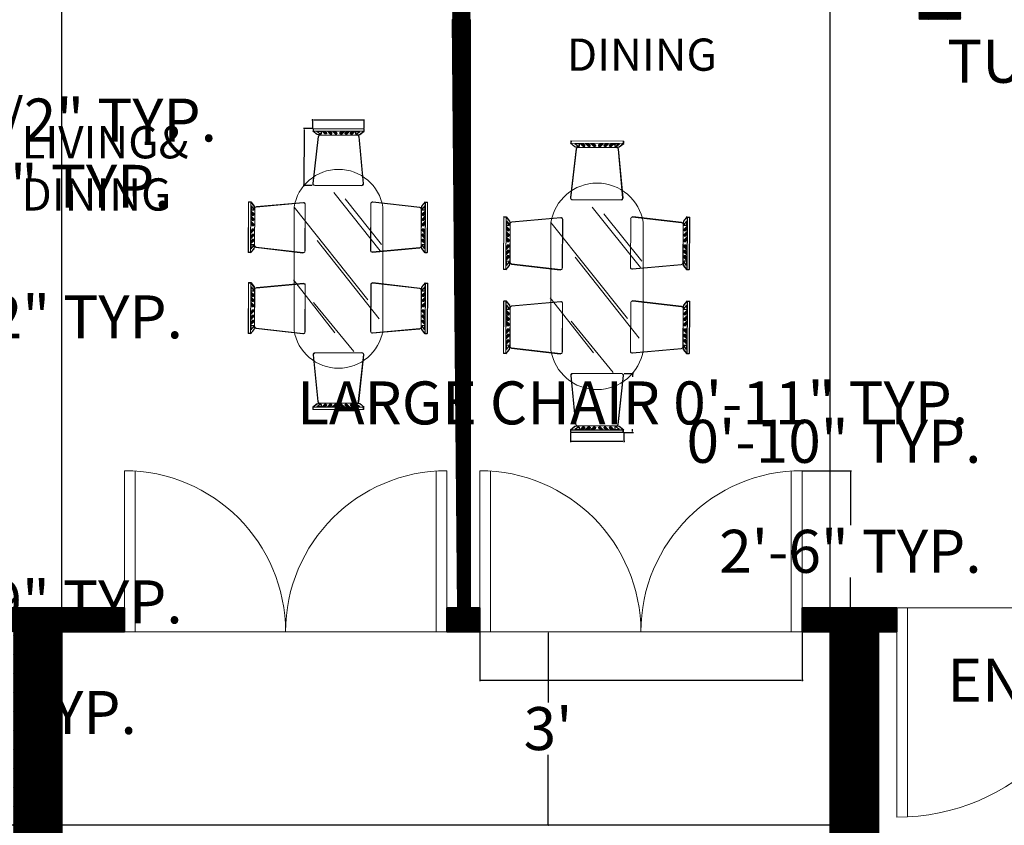
# Model space of a CAD drawing. Units: inches. Extents: x 108 to 771, y 58 to 590.
# Tile 4 of 8: x 341 to 524, y 253 to 402. Entities that reach past the tile are written whole.
import ezdxf

# ---------------------------------------------------------------- set-up
doc = ezdxf.new("R2010")
doc.units = ezdxf.units.IN
doc.header["$MEASUREMENT"] = 0
for name, color, linetype, lineweight in [('A-ANNO-DIMS', 2, 'Continuous', 13), ('A-AREA-IDEN', 7, 'Continuous', 18), ('A-DOOR', 3, 'Continuous', 18), ('A-WALL', 7, 'Continuous', 35), ('A-WALL-PATT', 252, 'Continuous', 9), ('Furniture', 7, 'Continuous', 15)]:
    doc.layers.add(name, color=color, linetype=linetype, lineweight=lineweight)
doc.styles.get("Standard").update_dxf_attribs({"font": 'italic8.shx'})
doc.dimstyles.get("Standard").update_dxf_attribs({"dimtxt": 8, "dimasz": 0.18, "dimexe": 0.18, "dimexo": 0.0625, "dimgap": 0.09, "dimtad": 0, "dimtih": 1, "dimtoh": 1, "dimzin": 0, "dimdsep": 46, "dimlunit": 3, "dimtxsty": 'Standard', "dimcen": 0.09, "dimclrt": 6, "dimadec": 0, "dimazin": 0, "dimtfac": 1, "dimtofl": 0, "dimtmove": 0, "dimatfit": 3, "dimfxl": 1, "dimtolj": 1, "dimtzin": 0, "dimarcsym": 0})

# ---------------------------------------------------------------- blocks, each defined once
blk = doc.blocks.new('*D3')
at = {"layer": 'A-ANNO-DIMS', "color": 0, "lineweight": -2, "transparency": 16777216}
for p, q in [((438.84, 288.37), (438.84, 275.4)), ((438.9, 288.55), (439.02, 288.55)), ((438.84, 252.73), (438.84, 265.7)), ((438.9, 252.55), (439.02, 252.55))]:
    blk.add_line(p, q, dxfattribs=at)
at = {"layer": 'A-ANNO-DIMS', "color": 0, "transparency": 16777216}
for points in [[(438.81, 288.37), (438.87, 288.37), (438.84, 288.55)], [(438.81, 252.73), (438.87, 252.73), (438.84, 252.55)]]:
    blk.add_solid(points, dxfattribs=at)
at = {"layer": 'Defpoints', "color": 0, "transparency": 16777216}
for p in [(438.84, 288.55), (438.84, 288.55), (438.84, 252.55)]:
    blk.add_point(p, dxfattribs=at)
at = {"layer": 'A-ANNO-DIMS', "color": 0, "transparency": 16777216, "insert": (438.84, 270.55), "char_height": 8, "attachment_point": 5}
blk.add_mtext("\\A1;3'", dxfattribs=at)
blk = doc.blocks.new('DOOR-SINGLE-39')
for p, q in [((0, 39), (0, 0)), ((2, 38.95), (2, 0)), ((0, 0), (39, 0))]:
    blk.add_line(p, q)
blk.add_arc((0, 0), 39, 0, 90)
blk = doc.blocks.new('DOOR-PAIR-60')
for p, q in [((0, 0), (0, 30)), ((2, 0), (2, 29.93)), ((58, 0), (58, 29.93)), ((60, 0), (60, 30)), ((0, 0), (60, 0))]:
    blk.add_line(p, q)
for centre, start, end in [((0, 0), 0, 90), ((60, 0), 90, 180)]:
    blk.add_arc(centre, 30, start, end)
blk = doc.blocks.new('DINING-CHAIR')
for p, q in [((0.9, 1.48), (0.06, 10.23)), ((0.99, 1.45), (0.14, 10.2)), ((0.38, 10.58), (9.09, 10.59)), ((0.46, 10.55), (9.17, 10.56)), ((9.41, 10.23), (8.46, 1.48)), ((9.49, 10.2), (8.54, 1.45)), ((0, 0.48), (0.8, 1.13)), ((9.39, 0.46), (0, 0.45)), ((0, 0.45), (0, 0.03)), ((0, 0.03), (9.39, 0.04)), ((0.08, 0.45), (0.89, 1.09)), ((9.48, 0.43), (0.08, 0.42)), ((0.08, 0.42), (0.08, 0)), ((0.08, 0), (9.48, 0.01)), ((1.48, 1.09), (0.77, 0.58)), ((0.77, 0.58), (1.54, 0.55)), ((0.8, 1.13), (1.48, 1.09)), ((1.56, 1.06), (0.85, 0.55)), ((0.85, 0.55), (1.63, 0.52)), ((0.89, 1.09), (1.56, 1.06)), ((8.14, 1.2), (1.22, 1.19)), ((8.22, 1.17), (1.31, 1.16)), ((1.54, 0.55), (1.51, 1)), ((1.63, 0.52), (1.59, 0.97)), ((1.74, 0.51), (2.22, 1)), ((1.82, 0.48), (2.3, 0.97)), ((2.48, 1), (1.99, 0.55)), ((1.99, 0.55), (2.19, 0.55)), ((2.56, 0.97), (2.08, 0.52)), ((2.08, 0.52), (2.27, 0.52)), ((2.19, 0.55), (2.41, 0.74)), ((2.22, 1), (2.48, 1)), ((2.27, 0.52), (2.5, 0.71)), ((2.3, 0.97), (2.56, 0.97)), ((2.41, 0.74), (2.48, 0.68)), ((2.48, 0.68), (2.51, 0.97)), ((2.5, 0.71), (2.56, 0.65)), ((2.56, 0.65), (2.59, 0.94)), ((2.7, 0.52), (3.18, 1)), ((2.79, 0.49), (3.27, 0.97)), ((3.44, 1), (2.96, 0.55)), ((2.96, 0.55), (3.15, 0.55)), ((3.52, 0.97), (3.04, 0.52)), ((3.04, 0.52), (3.24, 0.52)), ((3.15, 0.55), (3.38, 0.74)), ((3.18, 1), (3.44, 1)), ((3.24, 0.52), (3.46, 0.71)), ((3.27, 0.97), (3.52, 0.97)), ((3.38, 0.74), (3.44, 0.68)), ((3.44, 0.68), (3.47, 0.97)), ((3.46, 0.71), (3.53, 0.65)), ((3.53, 0.65), (3.56, 0.94)), ((3.67, 0.52), (4.15, 1)), ((3.75, 0.49), (4.23, 0.97)), ((4.41, 1), (3.92, 0.55)), ((3.92, 0.55), (4.12, 0.55)), ((4.49, 0.97), (4.01, 0.52)), ((4.01, 0.52), (4.2, 0.52)), ((4.12, 0.55), (4.34, 0.74)), ((4.15, 1), (4.41, 1)), ((4.2, 0.52), (4.43, 0.71)), ((4.23, 0.97), (4.49, 0.97)), ((4.34, 0.74), (4.41, 0.68)), ((4.41, 0.68), (4.44, 0.97)), ((4.43, 0.71), (4.49, 0.65)), ((4.49, 0.65), (4.52, 0.94)), ((5.05, 0.68), (5.02, 0.97)), ((5.31, 1), (5.05, 1)), ((5.05, 1), (5.53, 0.55)), ((5.12, 0.74), (5.05, 0.68)), ((5.13, 0.65), (5.1, 0.94)), ((5.34, 0.55), (5.12, 0.74)), ((5.39, 0.97), (5.13, 0.97)), ((5.13, 0.97), (5.62, 0.52)), ((5.2, 0.71), (5.13, 0.65)), ((5.42, 0.52), (5.2, 0.71)), ((5.79, 0.52), (5.31, 1)), ((5.53, 0.55), (5.34, 0.55)), ((5.87, 0.49), (5.39, 0.97)), ((5.62, 0.52), (5.42, 0.52)), ((6.02, 0.68), (5.98, 0.97)), ((6.27, 1), (6.02, 1)), ((6.02, 1), (6.5, 0.55)), ((6.08, 0.74), (6.02, 0.68)), ((6.1, 0.65), (6.07, 0.94)), ((6.31, 0.55), (6.08, 0.74)), ((6.36, 0.97), (6.1, 0.97)), ((6.1, 0.97), (6.58, 0.52)), ((6.16, 0.71), (6.1, 0.65)), ((6.39, 0.52), (6.16, 0.71)), ((6.76, 0.52), (6.27, 1)), ((6.5, 0.55), (6.31, 0.55)), ((6.84, 0.49), (6.36, 0.97)), ((6.58, 0.52), (6.39, 0.52)), ((6.98, 0.68), (6.95, 0.97)), ((7.24, 1), (6.98, 1)), ((6.98, 1), (7.46, 0.55)), ((7.05, 0.74), (6.98, 0.68)), ((7.06, 0.65), (7.03, 0.94)), ((7.27, 0.55), (7.05, 0.74)), ((7.32, 0.97), (7.06, 0.97)), ((7.06, 0.97), (7.55, 0.52)), ((7.13, 0.71), (7.06, 0.65)), ((7.35, 0.52), (7.13, 0.71)), ((7.72, 0.52), (7.24, 1)), ((7.46, 0.55), (7.27, 0.55)), ((7.8, 0.49), (7.32, 0.97)), ((7.55, 0.52), (7.35, 0.52)), ((7.91, 0.55), (7.95, 1)), ((8.69, 0.59), (7.91, 0.55)), ((8.65, 1.13), (7.98, 1.1)), ((7.98, 1.1), (8.69, 0.59)), ((8, 0.52), (8.03, 0.97)), ((8.77, 0.55), (8, 0.52)), ((8.74, 1.1), (8.06, 1.07)), ((8.06, 1.07), (8.77, 0.55)), ((9.46, 0.49), (8.65, 1.13)), ((9.54, 0.46), (8.74, 1.1)), ((9.39, 0.04), (9.39, 0.46)), ((9.48, 0.01), (9.48, 0.43))]:
    blk.add_line(p, q)
for centre, start, end in [((0.38, 10.26), 90.0502, 185.5303), ((0.46, 10.23), 90.0502, 185.5303), ((9.09, 10.27), 353.7931, 90.0502), ((9.17, 10.23), 353.7931, 90.0502), ((1.22, 1.51), 185.5303, 270.0502), ((1.31, 1.48), 185.5303, 270.0502), ((8.14, 1.52), 270.0502, 353.7931), ((8.22, 1.49), 270.0502, 353.7931)]:
    blk.add_arc(centre, 0.322, start, end)
blk = doc.blocks.new('DINING-CHAIR-LARGE')
for p, q in [((0.94, 1.54), (0.06, 10.62)), ((1.02, 1.5), (0.15, 10.58)), ((0.39, 10.98), (9.44, 10.99)), ((0.48, 10.95), (9.52, 10.96)), ((9.77, 10.62), (8.78, 1.54)), ((9.86, 10.59), (8.87, 1.51)), ((0, 0.5), (0.83, 1.17)), ((9.75, 0.47), (0, 0.47)), ((0, 0.47), (0, 0.03)), ((0, 0.03), (9.75, 0.04)), ((0.09, 0.47), (0.92, 1.14)), ((9.84, 0.44), (0.09, 0.43)), ((0.09, 0.43), (0.09, 0)), ((0.09, 0), (9.84, 0.01)), ((1.54, 1.13), (0.8, 0.6)), ((0.8, 0.6), (1.6, 0.57)), ((0.83, 1.17), (1.54, 1.13)), ((1.62, 1.1), (0.89, 0.57)), ((0.89, 0.57), (1.69, 0.54)), ((0.92, 1.14), (1.62, 1.1)), ((8.45, 1.24), (1.27, 1.23)), ((8.54, 1.21), (1.36, 1.2)), ((1.6, 0.57), (1.57, 1.03)), ((1.69, 0.54), (1.66, 1)), ((1.8, 0.53), (2.3, 1.03)), ((1.89, 0.5), (2.39, 1)), ((2.57, 1.04), (2.07, 0.57)), ((2.07, 0.57), (2.27, 0.57)), ((2.66, 1), (2.16, 0.54)), ((2.16, 0.54), (2.36, 0.54)), ((2.27, 0.57), (2.5, 0.77)), ((2.3, 1.03), (2.57, 1.04)), ((2.36, 0.54), (2.59, 0.74)), ((2.39, 1), (2.66, 1)), ((2.5, 0.77), (2.57, 0.7)), ((2.57, 0.7), (2.6, 1)), ((2.59, 0.74), (2.66, 0.67)), ((2.66, 0.67), (2.69, 0.97)), ((2.81, 0.53), (3.31, 1.04)), ((2.89, 0.5), (3.39, 1)), ((3.57, 1.04), (3.07, 0.57)), ((3.07, 0.57), (3.27, 0.57)), ((3.66, 1), (3.16, 0.54)), ((3.16, 0.54), (3.36, 0.54)), ((3.27, 0.57), (3.51, 0.77)), ((3.31, 1.04), (3.57, 1.04)), ((3.36, 0.54), (3.59, 0.74)), ((3.39, 1), (3.66, 1)), ((3.51, 0.77), (3.57, 0.7)), ((3.57, 0.7), (3.61, 1)), ((3.59, 0.74), (3.66, 0.67)), ((3.66, 0.67), (3.69, 0.97)), ((3.81, 0.54), (4.31, 1.04)), ((3.89, 0.5), (4.39, 1)), ((4.58, 1.04), (4.07, 0.57)), ((4.07, 0.57), (4.27, 0.57)), ((4.66, 1.01), (4.16, 0.54)), ((4.16, 0.54), (4.36, 0.54)), ((4.27, 0.57), (4.51, 0.77)), ((4.31, 1.04), (4.58, 1.04)), ((4.36, 0.54), (4.59, 0.74)), ((4.39, 1), (4.66, 1.01)), ((4.51, 0.77), (4.58, 0.7)), ((4.58, 0.7), (4.61, 1)), ((4.59, 0.74), (4.66, 0.67)), ((4.66, 0.67), (4.69, 0.97)), ((5.24, 0.7), (5.21, 1)), ((5.51, 1.04), (5.24, 1.04)), ((5.24, 1.04), (5.74, 0.57)), ((5.31, 0.77), (5.24, 0.7)), ((5.33, 0.67), (5.3, 0.97)), ((5.54, 0.57), (5.31, 0.77)), ((5.6, 1.01), (5.33, 1.01)), ((5.33, 1.01), (5.83, 0.54)), ((5.4, 0.74), (5.33, 0.67)), ((5.63, 0.54), (5.4, 0.74)), ((6.01, 0.54), (5.51, 1.04)), ((5.74, 0.57), (5.54, 0.57)), ((6.1, 0.51), (5.6, 1.01)), ((5.83, 0.54), (5.63, 0.54)), ((6.25, 0.7), (6.21, 1)), ((6.51, 1.04), (6.25, 1.04)), ((6.25, 1.04), (6.75, 0.57)), ((6.31, 0.77), (6.25, 0.7)), ((6.33, 0.67), (6.3, 0.97)), ((6.55, 0.57), (6.31, 0.77)), ((6.6, 1.01), (6.33, 1.01)), ((6.33, 1.01), (6.83, 0.54)), ((6.4, 0.74), (6.33, 0.67)), ((6.63, 0.54), (6.4, 0.74)), ((7.01, 0.54), (6.51, 1.04)), ((6.75, 0.57), (6.55, 0.57)), ((7.1, 0.51), (6.6, 1.01)), ((6.83, 0.54), (6.63, 0.54)), ((7.25, 0.71), (7.21, 1.01)), ((7.51, 1.04), (7.25, 1.04)), ((7.25, 1.04), (7.75, 0.57)), ((7.31, 0.77), (7.25, 0.71)), ((7.33, 0.67), (7.3, 0.97)), ((7.55, 0.57), (7.31, 0.77)), ((7.6, 1.01), (7.33, 1.01)), ((7.33, 1.01), (7.83, 0.54)), ((7.4, 0.74), (7.33, 0.67)), ((7.63, 0.54), (7.4, 0.74)), ((8.02, 0.54), (7.51, 1.04)), ((7.75, 0.57), (7.55, 0.57)), ((8.1, 0.51), (7.6, 1.01)), ((7.83, 0.54), (7.63, 0.54)), ((8.22, 0.57), (8.25, 1.04)), ((9.02, 0.61), (8.22, 0.57)), ((8.98, 1.17), (8.28, 1.14)), ((8.28, 1.14), (9.02, 0.61)), ((8.3, 0.54), (8.34, 1.01)), ((9.1, 0.58), (8.3, 0.54)), ((9.07, 1.14), (8.37, 1.11)), ((8.37, 1.11), (9.1, 0.58)), ((9.82, 0.51), (8.98, 1.17)), ((9.91, 0.48), (9.07, 1.14)), ((9.75, 0.04), (9.75, 0.47)), ((9.84, 0.01), (9.84, 0.44))]:
    blk.add_line(p, q)
for centre, start, end in [((0.39, 10.65), 90.0502, 185.5303), ((0.48, 10.62), 90.0502, 185.5303), ((9.44, 10.66), 353.7931, 90.0502), ((9.52, 10.62), 353.7931, 90.0502), ((1.27, 1.57), 185.5303, 270.0502), ((1.36, 1.54), 185.5303, 270.0502), ((8.45, 1.57), 270.0502, 353.7931), ((8.54, 1.54), 270.0502, 353.7931)]:
    blk.add_arc(centre, 0.334, start, end)
blk = doc.blocks.new('*D29')
at = {"layer": 'A-ANNO-DIMS', "color": 0, "lineweight": -2, "transparency": 16777216}
for p, q in [((332.1, 293.05), (338.07, 293.05)), ((337.89, 292.87), (337.89, 278.4)), ((337.89, 254.23), (337.89, 268.7)), ((332.1, 254.05), (338.07, 254.05))]:
    blk.add_line(p, q, dxfattribs=at)
at = {"layer": 'A-ANNO-DIMS', "color": 0, "transparency": 16777216}
for points in [[(337.86, 292.87), (337.92, 292.87), (337.89, 293.05)], [(337.86, 254.23), (337.92, 254.23), (337.89, 254.05)]]:
    blk.add_solid(points, dxfattribs=at)
at = {"layer": 'Defpoints', "color": 0, "transparency": 16777216}
for p in [(332.04, 293.05), (332.04, 254.05), (337.89, 254.05)]:
    blk.add_point(p, dxfattribs=at)
at = {"layer": 'A-ANNO-DIMS', "color": 6, "transparency": 16777216, "insert": (337.89, 273.55), "char_height": 8, "attachment_point": 5}
blk.add_mtext('\\A1;3\'-3" TYP.', dxfattribs=at)
blk = doc.blocks.new('*D30')
at = {"layer": 'A-ANNO-DIMS', "color": 0, "lineweight": -2, "transparency": 16777216}
for p, q in [((426.12, 288.49), (426.12, 279.37)), ((486.12, 288.49), (486.12, 279.37)), ((426.3, 279.55), (485.94, 279.55)), ((486.12, 279.55), (486.3, 279.55))]:
    blk.add_line(p, q, dxfattribs=at)
at = {"layer": 'A-ANNO-DIMS', "color": 0, "transparency": 16777216}
for points in [[(426.3, 279.58), (426.3, 279.52), (426.12, 279.55)], [(485.94, 279.58), (485.94, 279.52), (486.12, 279.55)]]:
    blk.add_solid(points, dxfattribs=at)
at = {"layer": 'Defpoints', "color": 0, "transparency": 16777216}
for p in [(426.12, 288.55), (486.12, 288.55), (486.12, 279.55)]:
    blk.add_point(p, dxfattribs=at)
at = {"layer": 'A-ANNO-DIMS', "color": 6, "transparency": 16777216, "insert": (568.68, 279.55), "char_height": 8, "attachment_point": 5}
blk.add_mtext('\\A1;ENTRY PAIR 5\'-0" TYP.', dxfattribs=at)
blk = doc.blocks.new('*D31')
at = {"layer": 'A-ANNO-DIMS', "color": 0, "lineweight": -2, "transparency": 16777216}
for p, q in [((486.19, 318.55), (495.3, 318.55)), ((495.12, 318.37), (495.12, 308.4)), ((495.12, 288.73), (495.12, 298.7)), ((486.19, 288.55), (495.3, 288.55))]:
    blk.add_line(p, q, dxfattribs=at)
at = {"layer": 'A-ANNO-DIMS', "color": 0, "transparency": 16777216}
for points in [[(495.09, 318.37), (495.15, 318.37), (495.12, 318.55)], [(495.09, 288.73), (495.15, 288.73), (495.12, 288.55)]]:
    blk.add_solid(points, dxfattribs=at)
at = {"layer": 'Defpoints', "color": 0, "transparency": 16777216}
for p in [(486.12, 318.55), (495.12, 318.55), (486.12, 288.55)]:
    blk.add_point(p, dxfattribs=at)
at = {"layer": 'A-ANNO-DIMS', "color": 6, "transparency": 16777216, "insert": (495.12, 303.55), "char_height": 8, "attachment_point": 5}
blk.add_mtext('\\A1;2\'-6" TYP.', dxfattribs=at)
blk = doc.blocks.new('*D32')
at = {"layer": 'A-ANNO-DIMS', "color": 0, "lineweight": -2, "transparency": 16777216}
for p, q in [((395.01, 382.23), (393.3, 382.24)), ((393.48, 382.06), (393.42, 371.84)), ((394.94, 371.65), (393.24, 371.66)), ((393.42, 371.48), (393.24, 371.48)), ((393.42, 371.66), (393.42, 371.48))]:
    blk.add_line(p, q, dxfattribs=at)
at = {"layer": 'A-ANNO-DIMS', "color": 0, "transparency": 16777216}
for points in [[(393.45, 382.06), (393.51, 382.06), (393.48, 382.24)], [(393.39, 371.84), (393.45, 371.84), (393.42, 371.66)]]:
    blk.add_solid(points, dxfattribs=at)
at = {"layer": 'Defpoints', "color": 0, "transparency": 16777216}
for p in [(395.07, 382.23), (393.42, 371.66), (395.01, 371.65)]:
    blk.add_point(p, dxfattribs=at)
at = {"layer": 'A-ANNO-DIMS', "color": 6, "transparency": 16777216, "insert": (314.67, 371.48), "char_height": 8, "attachment_point": 5}
blk.add_mtext('\\A1;CHAIR 0\'-10 1/2" TYP.', dxfattribs=at)
blk = doc.blocks.new('*D33')
at = {"layer": 'A-ANNO-DIMS', "color": 0, "lineweight": -2, "transparency": 16777216}
for p, q in [((395.08, 383.82), (394.9, 383.82)), ((395.07, 382.3), (395.08, 384)), ((404.44, 383.77), (395.26, 383.82)), ((404.61, 382.24), (404.62, 383.94))]:
    blk.add_line(p, q, dxfattribs=at)
at = {"layer": 'A-ANNO-DIMS', "color": 0, "transparency": 16777216}
for points in [[(395.26, 383.85), (395.26, 383.79), (395.08, 383.82)], [(404.44, 383.8), (404.44, 383.74), (404.62, 383.76)]]:
    blk.add_solid(points, dxfattribs=at)
at = {"layer": 'Defpoints', "color": 0, "transparency": 16777216}
for p in [(395.08, 383.82), (395.07, 382.23), (404.61, 382.18)]:
    blk.add_point(p, dxfattribs=at)
at = {"layer": 'A-ANNO-DIMS', "color": 6, "transparency": 16777216, "insert": (343.38, 383.82), "char_height": 8, "attachment_point": 5}
blk.add_mtext('\\A1;0\'-9 1/2" TYP.', dxfattribs=at)
blk = doc.blocks.new('*D34')
at = {"layer": 'A-ANNO-DIMS', "color": 0, "lineweight": -2, "transparency": 16777216}
for p, q in [((452.99, 336.66), (454.76, 336.66)), ((454.58, 336.48), (454.58, 336.02)), ((454.58, 325.85), (454.58, 326.31)), ((452.99, 325.67), (454.76, 325.67))]:
    blk.add_line(p, q, dxfattribs=at)
at = {"layer": 'A-ANNO-DIMS', "color": 0, "transparency": 16777216}
for points in [[(454.55, 336.48), (454.61, 336.48), (454.58, 336.66)], [(454.55, 325.85), (454.61, 325.85), (454.58, 325.67)]]:
    blk.add_solid(points, dxfattribs=at)
at = {"layer": 'Defpoints', "color": 0, "transparency": 16777216}
for p in [(452.93, 336.66), (454.58, 336.66), (452.93, 325.67)]:
    blk.add_point(p, dxfattribs=at)
at = {"layer": 'A-ANNO-DIMS', "color": 6, "transparency": 16777216, "insert": (454.58, 331.17), "char_height": 8, "attachment_point": 5}
blk.add_mtext('\\A1;LARGE CHAIR 0\'-11" TYP.', dxfattribs=at)
blk = doc.blocks.new('*D35')
at = {"layer": 'A-ANNO-DIMS', "color": 0, "lineweight": -2, "transparency": 16777216}
for p, q in [((443.03, 325.61), (443.03, 323.84)), ((452.93, 325.61), (452.93, 323.84)), ((443.21, 324.02), (452.75, 324.02)), ((452.93, 324.02), (453.11, 324.02))]:
    blk.add_line(p, q, dxfattribs=at)
at = {"layer": 'A-ANNO-DIMS', "color": 0, "transparency": 16777216}
for points in [[(443.21, 324.05), (443.21, 323.99), (443.03, 324.02)], [(452.75, 324.05), (452.75, 323.99), (452.93, 324.02)]]:
    blk.add_solid(points, dxfattribs=at)
at = {"layer": 'Defpoints', "color": 0, "transparency": 16777216}
for p in [(443.03, 325.67), (452.93, 325.67), (452.93, 324.02)]:
    blk.add_point(p, dxfattribs=at)
at = {"layer": 'A-ANNO-DIMS', "color": 6, "transparency": 16777216, "insert": (492.06, 324.02), "char_height": 8, "attachment_point": 5}
blk.add_mtext('\\A1;0\'-10" TYP.', dxfattribs=at)
blk = doc.blocks.new('*D38')
at = {"layer": 'A-ANNO-DIMS', "color": 0, "lineweight": -2, "transparency": 16777216}
for p, q in [((606.93, 394.75), (606.75, 394.75)), ((606.93, 385.95), (606.93, 394.93)), ((665.8, 394.75), (607.11, 394.75)), ((665.98, 385.95), (665.98, 394.93))]:
    blk.add_line(p, q, dxfattribs=at)
at = {"layer": 'A-ANNO-DIMS', "color": 0, "transparency": 16777216}
for points in [[(607.11, 394.78), (607.11, 394.72), (606.93, 394.75)], [(665.8, 394.78), (665.8, 394.72), (665.98, 394.75)]]:
    blk.add_solid(points, dxfattribs=at)
at = {"layer": 'Defpoints', "color": 0, "transparency": 16777216}
for p in [(606.93, 394.75), (606.93, 385.89), (665.98, 385.89)]:
    blk.add_point(p, dxfattribs=at)
at = {"layer": 'A-ANNO-DIMS', "color": 6, "transparency": 16777216, "insert": (552.56, 394.75), "char_height": 8, "attachment_point": 5}
blk.add_mtext('\\A1;TUB 4\'-11" TYP.', dxfattribs=at)
blk = doc.blocks.new('*D44')
at = {"layer": 'A-ANNO-DIMS', "color": 0, "lineweight": -2, "transparency": 16777216}
for p, q in [((310.02, 387.98), (322.38, 387.98)), ((322.2, 387.8), (322.2, 353.37)), ((322.2, 306.56), (322.2, 341)), ((310.02, 306.38), (322.38, 306.38))]:
    blk.add_line(p, q, dxfattribs=at)
at = {"layer": 'A-ANNO-DIMS', "color": 0, "transparency": 16777216}
for points in [[(322.17, 387.8), (322.23, 387.8), (322.2, 387.98)], [(322.17, 306.56), (322.23, 306.56), (322.2, 306.38)]]:
    blk.add_solid(points, dxfattribs=at)
at = {"layer": 'Defpoints', "color": 0, "transparency": 16777216}
for p in [(309.96, 387.98), (322.2, 387.98), (309.96, 306.38)]:
    blk.add_point(p, dxfattribs=at)
at = {"layer": 'A-ANNO-DIMS', "color": 6, "transparency": 16777216, "insert": (322.2, 347.18), "char_height": 8, "attachment_point": 5}
blk.add_mtext('\\A1;SOFA 6\'-9 1/2" TYP.', dxfattribs=at)
blk = doc.blocks.new('*D45')
at = {"layer": 'A-ANNO-DIMS', "color": 0, "lineweight": -2, "transparency": 16777216}
for p, q in [((277.12, 306.32), (277.12, 293.96)), ((309.96, 306.32), (309.96, 293.96)), ((277.3, 294.14), (309.78, 294.14)), ((309.96, 294.14), (310.14, 294.14))]:
    blk.add_line(p, q, dxfattribs=at)
at = {"layer": 'A-ANNO-DIMS', "color": 0, "transparency": 16777216}
for points in [[(277.3, 294.17), (277.3, 294.11), (277.12, 294.14)], [(309.78, 294.17), (309.78, 294.11), (309.96, 294.14)]]:
    blk.add_solid(points, dxfattribs=at)
at = {"layer": 'Defpoints', "color": 0, "transparency": 16777216}
for p in [(277.12, 306.38), (309.96, 306.38), (309.96, 294.14)]:
    blk.add_point(p, dxfattribs=at)
at = {"layer": 'A-ANNO-DIMS', "color": 6, "transparency": 16777216, "insert": (346.42, 294.14), "char_height": 8, "attachment_point": 5}
blk.add_mtext('\\A1;2\'-9" TYP.', dxfattribs=at)
blk = doc.blocks.new('*D52')
at = {"layer": 'A-ANNO-DIMS', "color": 0, "lineweight": -2, "transparency": 16777216}
for p, q in [((348.35, 145.12), (348.35, 578.33)), ((348.53, 578.15), (399.37, 578.15)), ((491.17, 578.15), (440.32, 578.15)), ((491.35, 145.12), (491.35, 578.33))]:
    blk.add_line(p, q, dxfattribs=at)
at = {"layer": 'A-ANNO-DIMS', "color": 0, "transparency": 16777216}
for points in [[(348.53, 578.18), (348.53, 578.12), (348.35, 578.15)], [(491.17, 578.18), (491.17, 578.12), (491.35, 578.15)]]:
    blk.add_solid(points, dxfattribs=at)
at = {"layer": 'Defpoints', "color": 0, "transparency": 16777216}
for p in [(491.35, 578.15), (348.35, 145.05), (491.35, 145.05)]:
    blk.add_point(p, dxfattribs=at)
at = {"layer": 'A-ANNO-DIMS', "color": 6, "transparency": 16777216, "insert": (419.85, 578.15), "char_height": 8, "attachment_point": 5}
blk.add_mtext('\\A1;11\'-11"', dxfattribs=at)
blk = doc.blocks.new('*D59')
at = {"layer": 'A-ANNO-DIMS', "color": 0, "lineweight": -2, "transparency": 16777216}
for p, q in [((327.35, 538.99), (327.35, 69.77)), ((331.85, 538.99), (331.85, 69.77)), ((327.53, 69.95), (331.67, 69.95)), ((331.85, 69.95), (332.03, 69.95))]:
    blk.add_line(p, q, dxfattribs=at)
at = {"layer": 'A-ANNO-DIMS', "color": 0, "transparency": 16777216}
for points in [[(327.53, 69.98), (327.53, 69.92), (327.35, 69.95)], [(331.67, 69.98), (331.67, 69.92), (331.85, 69.95)]]:
    blk.add_solid(points, dxfattribs=at)
at = {"layer": 'Defpoints', "color": 0, "transparency": 16777216}
for p in [(327.35, 539.05), (331.85, 539.05), (331.85, 69.95)]:
    blk.add_point(p, dxfattribs=at)
at = {"layer": 'A-ANNO-DIMS', "color": 6, "transparency": 16777216, "insert": (365.26, 69.95), "char_height": 8, "attachment_point": 5}
blk.add_mtext('\\A1;0\'-4 1/2"', dxfattribs=at)
blk = doc.blocks.new('*D61')
at = {"layer": 'A-ANNO-DIMS', "color": 0, "lineweight": -2, "transparency": 16777216}
for p, q in [((132.245389, 252.733083), (132.245389, 252.913083)), ((491.282889, 252.553083), (132.065389, 252.553083)), ((491.282889, 242.553083), (132.065389, 242.553083)), ((132.245389, 242.373083), (132.245389, 242.193083))]:
    blk.add_line(p, q, dxfattribs=at)
at = {"layer": 'A-ANNO-DIMS', "color": 0, "transparency": 16777216}
for points in [[(132.215389, 252.733083), (132.275389, 252.733083), (132.245389, 252.553083)], [(132.215389, 242.373083), (132.275389, 242.373083), (132.245389, 242.553083)]]:
    blk.add_solid(points, dxfattribs=at)
at = {"layer": 'Defpoints', "color": 0, "transparency": 16777216}
for p in [(491.345389, 252.553083), (132.245389, 242.553083), (491.345389, 242.553083)]:
    blk.add_point(p, dxfattribs=at)
at = {"layer": 'A-ANNO-DIMS', "color": 6, "transparency": 16777216, "insert": (132.245389, 247.553083), "char_height": 8, "attachment_point": 5}
blk.add_mtext('\\A1;0\'-10"', dxfattribs=at)

msp = doc.modelspace()

# ---------------------------------------------------------------- hatches: boundary and pattern name
at = {"layer": 'A-WALL-PATT'}
h = msp.add_hatch(dxfattribs=at)
h.set_pattern_fill('ANSI31', color=256)
h.paths.add_polyline_path([(171.345, 461.548), (162.345, 461.548), (162.345, 390.901), (171.345, 390.901), (171.345, 393.51), (171.345, 402.553), (233.142, 402.553), (233.142, 407.053), (171.345, 407.053)])
h.paths.add_polyline_path([(331.845, 438.553), (336.68, 438.554), (336.68, 443.053), (331.845, 443.053), (331.845, 539.053), (365.02, 539.053), (365.02, 548.053), (280.772, 548.053), (280.772, 539.053), (327.345, 539.053), (327.345, 407.053), (325.63, 407.053), (325.63, 402.553), (331.845, 402.553)])
h.paths.add_polyline_path([(286.63, 407.053), (263.142, 407.053), (263.142, 402.553), (267.345, 402.553), (267.345, 352.303), (171.345, 352.303), (171.345, 360.901), (162.345, 360.901), (162.345, 336.026), (171.345, 336.026), (171.345, 347.803), (267.345, 347.803), (267.345, 293.053), (263.142, 293.053), (263.142, 288.553), (293.037, 288.553), (293.037, 293.053), (271.845, 293.053), (271.845, 402.553), (286.63, 402.553)])
h.paths.add_polyline_path([(466.018, 443.053), (424.345, 443.053), (424.345, 539.053), (453.584, 539.053), (453.584, 548.053), (395.02, 548.053), (395.02, 539.053), (419.845, 539.053), (420.71, 443.053), (372.68, 443.053), (372.68, 438.557), (420.751, 438.561), (421.075, 402.553), (422.061, 293.053), (419.994, 293.053), (419.994, 288.553), (426.124, 288.553), (426.124, 293.053), (424.345, 293.053), (424.345, 402.553), (424.345, 438.553), (466.018, 438.553)])
h.paths.add_polyline_path([(512.345, 539.053), (583.918, 539.053), (583.918, 548.053), (483.584, 548.053), (483.584, 539.053), (507.845, 539.053), (507.845, 443.053), (502.018, 443.053), (502.018, 438.553), (507.845, 438.553), (507.845, 402.553), (515.658, 402.553), (515.658, 407.053), (512.345, 407.053)])
h.paths.add_polyline_path([(232.772, 548.053), (162.345, 548.053), (162.345, 509.548), (171.345, 509.548), (171.345, 539.053), (232.772, 539.053)])
h.paths.add_polyline_path([(233.142, 293.053), (171.345, 293.053), (171.345, 306.026), (162.345, 306.026), (162.345, 230.8), (171.345, 230.8), (171.345, 288.553), (233.142, 288.553)])
h.paths.add_polyline_path([(359.994, 293.053), (332.037, 293.053), (332.037, 288.553), (339.345, 288.553), (339.345, 145.053), (334.469, 145.053), (334.469, 136.053), (339.345, 136.053), (339.345, 104.553), (166.845, 104.553), (166.845, 136.053), (211.837, 136.053), (211.837, 145.053), (171.345, 145.053), (171.345, 182.8), (162.345, 182.8), (162.345, 100.053), (343.845, 100.053), (343.845, 136.053), (400.886, 136.053), (400.886, 145.053), (348.345, 145.053), (348.345, 288.553), (359.994, 288.553)])
h.paths.add_polyline_path([(500.345, 288.553), (503.755, 288.553), (503.755, 293.053), (486.124, 293.053), (486.124, 288.553), (491.345, 288.553), (491.345, 145.053), (448.886, 145.053), (448.886, 136.053), (495.845, 136.053), (495.845, 100.053), (677.345, 100.053), (677.345, 186.265), (668.345, 186.265), (668.345, 145.053), (627.637, 145.053), (627.637, 136.053), (672.845, 136.053), (672.845, 104.278), (500.345, 104.539), (500.345, 136.053), (504.239, 136.053), (504.239, 145.053), (500.345, 145.053)])
h.paths.add_polyline_path([(580.913, 293.053), (572.345, 293.053), (572.345, 347.803), (668.345, 347.803), (668.345, 330.831), (677.345, 330.831), (677.345, 366.853), (668.345, 366.853), (668.345, 352.303), (572.345, 352.303), (572.345, 402.553), (580.418, 402.553), (580.418, 407.053), (554.658, 407.053), (554.658, 402.553), (567.845, 402.553), (567.845, 293.053), (542.755, 293.053), (542.755, 288.553), (580.913, 288.553)])
h.paths.add_polyline_path([(677.345, 300.831), (668.345, 300.831), (668.345, 293.053), (610.913, 293.053), (610.913, 288.553), (668.345, 288.553), (668.345, 234.265), (677.345, 234.265)])
h.paths.add_polyline_path([(304.469, 145.053), (259.837, 145.053), (259.837, 136.053), (304.469, 136.053)], flags=17)
h.paths.add_polyline_path([(579.637, 145.053), (534.239, 145.053), (534.239, 136.053), (579.637, 136.053)], flags=17)
h.paths.add_polyline_path([(677.345, 450.416), (668.345, 450.416), (668.345, 407.053), (610.418, 407.053), (610.418, 402.553), (668.345, 402.553), (668.345, 396.853), (677.345, 396.853)])
h.paths.add_polyline_path([(677.345, 548.053), (631.918, 548.053), (631.918, 539.053), (668.345, 539.053), (668.345, 498.416), (677.345, 498.416)])
h = msp.add_hatch(dxfattribs=at)
h.set_pattern_fill('ANSI31', color=256)
h.paths.add_polyline_path([(365.02, 548.053), (280.772, 548.053), (280.772, 539.053), (327.345, 539.053), (327.345, 407.053), (325.63, 407.053), (325.63, 402.553), (331.845, 402.553), (331.845, 438.553), (336.68, 438.554), (336.68, 443.053), (331.845, 443.053), (331.845, 539.053), (365.02, 539.053)])
h.paths.add_polyline_path([(453.584, 548.053), (395.02, 548.053), (395.02, 539.053), (419.845, 539.053), (420.71, 443.053), (372.68, 443.053), (372.68, 438.557), (420.751, 438.561), (421.075, 402.553), (422.061, 293.053), (419.994, 293.053), (419.994, 288.553), (426.124, 288.553), (426.124, 293.053), (424.345, 293.053), (424.345, 402.553), (424.345, 438.553), (466.018, 438.553), (466.018, 443.053), (424.345, 443.053), (424.345, 539.053), (453.584, 539.053)])
h.paths.add_polyline_path([(232.772, 548.053), (162.345, 548.053), (162.345, 509.548), (171.345, 509.548), (171.345, 539.053), (232.772, 539.053)])
h.paths.add_polyline_path([(171.345, 461.548), (162.345, 461.548), (162.345, 390.901), (171.345, 390.901), (171.345, 393.51), (171.345, 402.553), (233.142, 402.553), (233.142, 407.053), (171.345, 407.053)])
h.paths.add_polyline_path([(286.63, 407.053), (263.142, 407.053), (263.142, 402.553), (267.345, 402.553), (267.345, 352.303), (171.345, 352.303), (171.345, 360.901), (162.345, 360.901), (162.345, 336.026), (171.345, 336.026), (171.345, 347.803), (267.345, 347.803), (267.345, 293.053), (263.142, 293.053), (263.142, 288.553), (293.037, 288.553), (293.037, 293.053), (271.845, 293.053), (271.845, 402.553), (286.63, 402.553)])
h.paths.add_polyline_path([(171.345, 306.026), (162.345, 306.026), (162.345, 230.8), (171.345, 230.8), (171.345, 288.553), (233.142, 288.553), (233.142, 293.053), (171.345, 293.053)])
h.paths.add_polyline_path([(348.345, 288.553), (359.994, 288.553), (359.994, 293.053), (332.037, 293.053), (332.037, 288.553), (339.345, 288.553), (339.345, 145.053), (334.469, 145.053), (334.469, 136.053), (339.345, 136.053), (339.345, 104.553), (166.845, 104.553), (166.845, 136.053), (211.837, 136.053), (211.837, 145.053), (171.345, 145.053), (171.345, 182.8), (162.345, 182.8), (162.345, 100.053), (343.845, 100.053), (343.845, 136.053), (400.886, 136.053), (400.886, 145.053), (348.345, 145.053)])
h.paths.add_polyline_path([(503.755, 293.053), (486.124, 293.053), (486.124, 288.553), (491.345, 288.553), (491.345, 145.053), (448.886, 145.053), (448.886, 136.053), (495.845, 136.053), (495.845, 100.053), (677.345, 100.053), (677.345, 186.265), (668.345, 186.265), (668.345, 145.053), (627.637, 145.053), (627.637, 136.053), (672.845, 136.053), (672.845, 104.278), (500.345, 104.539), (500.345, 136.053), (504.239, 136.053), (504.239, 145.053), (500.345, 145.053), (500.345, 288.553), (503.755, 288.553)])
h.paths.add_polyline_path([(580.913, 293.053), (572.345, 293.053), (572.345, 347.803), (668.345, 347.803), (668.345, 330.831), (677.345, 330.831), (677.345, 366.853), (668.345, 366.853), (668.345, 352.303), (572.345, 352.303), (572.345, 402.553), (580.418, 402.553), (580.418, 407.053), (554.658, 407.053), (554.658, 402.553), (567.845, 402.553), (567.845, 293.053), (542.755, 293.053), (542.755, 288.553), (580.913, 288.553)])
h.paths.add_polyline_path([(677.345, 300.831), (668.345, 300.831), (668.345, 293.053), (610.913, 293.053), (610.913, 288.553), (668.345, 288.553), (668.345, 234.265), (677.345, 234.265)])
h.paths.add_polyline_path([(579.637, 145.053), (534.239, 145.053), (534.239, 136.053), (579.637, 136.053)], flags=17)
h.paths.add_polyline_path([(304.469, 145.053), (259.837, 145.053), (259.837, 136.053), (304.469, 136.053)], flags=17)
h.paths.add_polyline_path([(583.918, 548.053), (483.584, 548.053), (483.584, 539.053), (507.845, 539.053), (507.845, 443.053), (502.018, 443.053), (502.018, 438.553), (507.845, 438.553), (507.845, 402.553), (515.658, 402.553), (515.658, 407.053), (512.345, 407.053), (512.345, 539.053), (583.918, 539.053)])
h.paths.add_polyline_path([(677.345, 548.053), (631.918, 548.053), (631.918, 539.053), (668.345, 539.053), (668.345, 498.416), (677.345, 498.416)])
h.paths.add_polyline_path([(677.345, 450.416), (668.345, 450.416), (668.345, 407.053), (610.418, 407.053), (610.418, 402.553), (668.345, 402.553), (668.345, 396.853), (677.345, 396.853)])

# ---------------------------------------------------------------- linework, layer by layer
at = {"layer": 'A-WALL'}
for p, q in [((422.061, 293.053), (421.075, 402.553)), ((424.345, 293.053), (424.345, 402.553)), ((359.994, 293.053), (332.037, 293.053)), ((359.994, 293.053), (359.994, 288.553)), ((422.061, 293.053), (419.994, 293.053)), ((419.994, 293.053), (419.994, 288.553)), ((426.124, 293.053), (424.345, 293.053)), ((426.124, 288.553), (426.124, 293.053)), ((486.124, 288.553), (486.124, 293.053)), ((503.755, 293.053), (486.124, 293.053)), ((503.755, 288.553), (503.755, 293.053)), ((348.345, 145.053), (348.345, 288.553)), ((359.994, 288.553), (348.345, 288.553)), ((426.124, 288.553), (419.994, 288.553)), ((491.345, 288.553), (486.124, 288.553)), ((491.345, 288.553), (491.345, 145.053)), ((500.345, 288.553), (500.345, 145.053)), ((503.755, 288.553), (500.345, 288.553))]:
    msp.add_line(p, q, dxfattribs=at)
at = {"layer": 'Furniture'}
for p, q in [((398.945, 370.301, 1.829), (407.624, 359.498, 1.829)), ((401.056, 369.126, 1.829), (407.858, 360.672, 1.829)), ((391.564, 367.587, 1.829), (405.278, 350.339, 1.829)), ((391.564, 367.587, 1.829), (391.564, 344.672, 1.829)), ((408.12, 344.672, 1.829), (408.12, 367.587, 1.829)), ((447.048, 367.575, 1.899), (456.057, 356.361, 1.899)), ((439.385, 364.758, 1.899), (453.622, 346.853, 1.899)), ((439.385, 364.758, 1.899), (439.385, 340.971, 1.899)), ((449.239, 366.356, 1.899), (456.3, 357.58, 1.899)), ((456.572, 340.971, 1.899), (456.572, 364.758, 1.899)), ((395.896, 361.377, 1.829), (407.389, 346.816, 1.829)), ((443.882, 358.311, 1.899), (455.813, 343.196, 1.899)), ((391.439, 354.096, 1.829), (399.179, 344.233, 1.829)), ((439.256, 350.754, 1.899), (447.291, 340.515, 1.899)), ((395.192, 349.869, 1.829), (402.698, 340.71, 1.829)), ((443.152, 346.366, 1.899), (450.943, 336.858, 1.899))]:
    msp.add_line(p, q, dxfattribs=at)
for centre, radius, start, end in [((399.842, 366.256, 1.829), 8.384, 9.13208, 170.86792), ((447.979, 363.376, 1.899), 8.704, 9.13208, 170.86792), ((399.842, 346.003, 1.829), 8.384, 189.13208, 350.86792), ((447.979, 342.352, 1.899), 8.704, 189.13208, 350.86792)]:
    msp.add_arc(centre, radius, start, end, dxfattribs=at)

# ---------------------------------------------------------------- block references
at = {"layer": 'A-DOOR'}
for p in [(359.994, 288.553), (426.124, 288.553)]:
    msp.add_blockref('DOOR-PAIR-60', p, dxfattribs=at)
at = {"layer": 'A-DOOR', "extrusion": (0, 0, -1), "zscale": -1, "rotation": 180}
msp.add_blockref('DOOR-SINGLE-39', (-503.755, 293.053), dxfattribs=at)
at = {"layer": 'Furniture'}
for name, p, rotation in [('DINING-CHAIR', (404.612, 382.177), 179.6597344209331), ('DINING-CHAIR-LARGE', (452.93, 379.902), 179.6597344209245), ('DINING-CHAIR', (383.091, 368.623), 269.5985218114716), ('DINING-CHAIR', (416.398, 359.074), 89.70995657529639), ('DINING-CHAIR-LARGE', (430.591, 365.834), 269.5985218114689), ('DINING-CHAIR-LARGE', (465.165, 355.921), 89.70995657528844), ('DINING-CHAIR', (383.079, 353.553), 269.6597344209209), ('DINING-CHAIR', (416.4, 344.004), 89.64874396583393), ('DINING-CHAIR-LARGE', (430.579, 350.19), 269.659734420916), ('DINING-CHAIR-LARGE', (465.166, 340.277), 89.648743965827)]:
    msp.add_blockref(name, p, dxfattribs=dict(at, rotation=rotation))
for name, p in [('DINING-CHAIR', (395.072, 329.933)), ('DINING-CHAIR-LARGE', (443.027, 325.671))]:
    msp.add_blockref(name, p, dxfattribs=at)

# ---------------------------------------------------------------- texts
at = {"layer": 'A-AREA-IDEN'}
for s, p in [('DINING', (442.356, 392.987)), ('LIVING&', (340.843, 376.677)), ('DINING', (340.843, 366.962))]:
    msp.add_text(s, height=6, dxfattribs=at).set_placement(p)

# ---------------------------------------------------------------- dimensions: what is measured, and where the dimension line sits
at = {"layer": 'A-ANNO-DIMS'}
for base, p1, p2, picture, middle in [((491.345, 578.153), (348.345, 145.053), (491.345, 145.053), '*D52', (419.845, 578.153)), ((331.845, 69.953), (327.345, 539.053), (331.845, 539.053), '*D59', (365.258, 69.953))]:
    dim = msp.add_linear_dim(base=base, p1=p1, p2=p2, dimstyle='Standard', override={"dimdec": 1, "dimlfac": 1, "dimrnd": 0, "dimzin": 1, "dimdsep": 46, "dimlunit": 4, "dimfrac": 2}, dxfattribs=at)
    dim.commit()
    dim.dimension.update_dxf_attribs({"geometry": picture, "text_midpoint": middle})
for base, p1, p2, angle, text, picture, middle in [((606.926, 394.75), (665.981, 385.892), (606.926, 385.892), 180, 'TUB <> TYP.', '*D38', (552.561, 394.75)), ((395.079, 383.821), (404.612, 382.176), (395.07, 382.233), 179.65973, '<> TYP.', '*D33', (343.381, 383.822)), ((393.419, 371.656), (395.07, 382.233), (395.007, 371.646), 269.65973, 'CHAIR <> TYP.', '*D32', (314.672, 371.476)), ((322.202, 387.98), (309.962, 306.382), (309.962, 387.98), 90, 'SOFA <> TYP.', '*D44', (322.202, 347.181)), ((454.581, 336.66), (452.932, 325.671), (452.932, 336.66), 90, 'LARGE CHAIR <> TYP.', '*D34', (454.581, 331.166)), ((495.124, 318.553), (486.124, 288.553), (486.124, 318.553), 90, '<> TYP.', '*D31', (495.124, 303.553)), ((337.887, 254.053), (332.037, 293.053), (332.037, 254.053), 270, '<> TYP.', '*D29', (337.887, 273.553))]:
    dim = msp.add_linear_dim(base=base, p1=p1, p2=p2, angle=angle, text=text, dimstyle='Standard', override={"dimdec": 1, "dimlfac": 1, "dimrnd": 0, "dimzin": 1, "dimdsep": 46, "dimlunit": 4, "dimfrac": 2}, dxfattribs=at)
    dim.commit()
    dim.dimension.update_dxf_attribs({"geometry": picture, "text_midpoint": middle})
for base, p1, p2, text, picture, middle in [((452.932, 324.022), (443.027, 325.671), (452.932, 325.671), '<> TYP.', '*D35', (492.06, 324.022)), ((309.962, 294.142), (277.117, 306.382), (309.962, 306.382), '<> TYP.', '*D45', (346.422, 294.142)), ((486.124, 279.553), (426.124, 288.553), (486.124, 288.553), 'ENTRY PAIR <> TYP.', '*D30', (568.679, 279.553))]:
    dim = msp.add_linear_dim(base=base, p1=p1, p2=p2, text=text, dimstyle='Standard', override={"dimdec": 1, "dimlfac": 1, "dimrnd": 0, "dimzin": 1, "dimdsep": 46, "dimlunit": 4, "dimfrac": 2}, dxfattribs=at)
    dim.commit()
    dim.dimension.update_dxf_attribs({"geometry": picture, "text_midpoint": middle})
for base, p1, p2, override, picture, middle in [((438.84, 288.553), (438.84, 252.553), (438.84, 288.553), {"dimclrd": 0, "dimclre": 0, "dimclrt": 0}, '*D3', (438.84, 270.553)), ((132.245, 242.553), (491.345, 252.553), (491.345, 242.553), {"dimdec": 1, "dimlfac": 1, "dimrnd": 0, "dimzin": 1, "dimdsep": 46, "dimlunit": 4, "dimfrac": 2}, '*D61', (132.245, 247.553))]:
    dim = msp.add_linear_dim(base=base, p1=p1, p2=p2, angle=90, dimstyle='Standard', override=override, dxfattribs=at)
    dim.commit()
    dim.dimension.update_dxf_attribs({"geometry": picture, "text_midpoint": middle})

doc.saveas('drawing.dxf')
